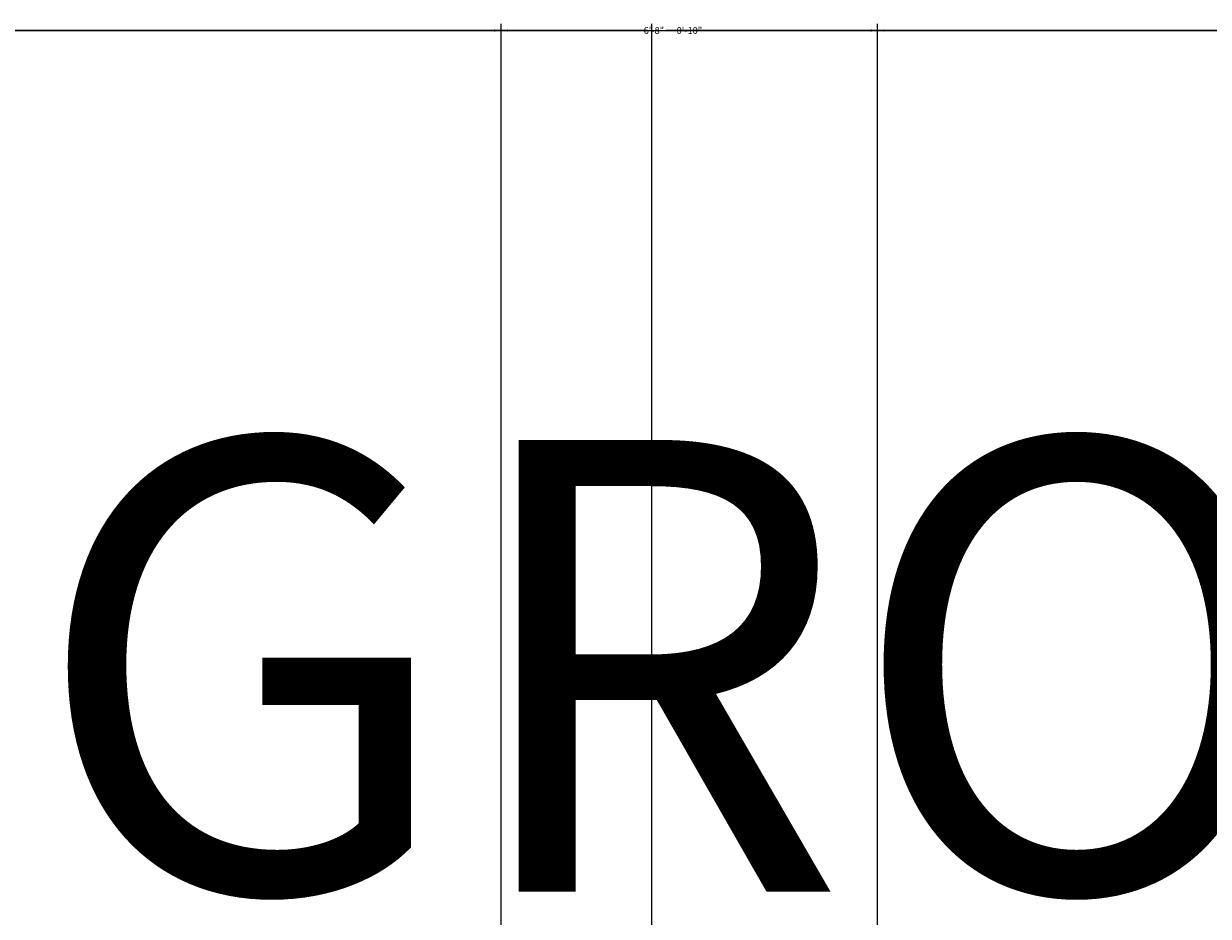
# Model space of a CAD drawing. Units: inches. Extents: x 37 to 824, y -700 to 234.
# Tile 59 of 77: x 193 to 225, y 210 to 234. Entities that reach past the tile are written whole.
import ezdxf

# ---------------------------------------------------------------- set-up
doc = ezdxf.new("R2010")
doc.units = ezdxf.units.IN
doc.header["$MEASUREMENT"] = 0
doc.layers.add('A-ANNO-DIMS', color=2, linetype='Continuous', lineweight=18)
doc.layers.add('A-ANNO-TEXT', color=7, linetype='Continuous', lineweight=18)
doc.styles.get("Standard").update_dxf_attribs({"font": 'arial.ttf'})
doc.dimstyles.get("Standard").update_dxf_attribs({"dimtxt": 0.18, "dimasz": 0.18, "dimexe": 0.18, "dimexo": 0.0625, "dimgap": 0.09, "dimtad": 0, "dimtih": 1, "dimtoh": 1, "dimdec": 1, "dimzin": 0, "dimdsep": 46, "dimlunit": 4, "dimtxsty": 'Standard', "dimcen": 0.09, "dimadec": 0, "dimazin": 0, "dimtfac": 1, "dimtdec": 1, "dimtofl": 0, "dimtmove": 0, "dimatfit": 3, "dimfxl": 1, "dimtolj": 1, "dimtzin": 0, "dimarcsym": 0})

# ---------------------------------------------------------------- blocks, each defined once
blk = doc.blocks.new('*D44')
at = {"layer": 'A-ANNO-DIMS', "color": 0, "lineweight": -2, "ltscale": 0.5, "transparency": 16777216}
for p, q in [((161.077, 191.153), (161.077, 234.17)), ((210.077, 191.153), (210.077, 234.17)), ((161.257, 233.99), (185.244, 233.99)), ((209.897, 233.99), (185.91, 233.99))]:
    blk.add_line(p, q, dxfattribs=at)
at = {"layer": 'A-ANNO-DIMS', "color": 0, "ltscale": 0.5, "transparency": 16777216}
for points in [[(161.257, 234.02), (161.257, 233.96), (161.077, 233.99)], [(209.897, 234.02), (209.897, 233.96), (210.077, 233.99)]]:
    blk.add_solid(points, dxfattribs=at)
at = {"layer": 'Defpoints', "color": 0, "ltscale": 0.5, "transparency": 16777216}
for p in [(210.077, 233.99), (161.077, 191.09), (210.077, 191.09)]:
    blk.add_point(p, dxfattribs=at)
at = {"layer": 'A-ANNO-DIMS', "color": 0, "ltscale": 0.5, "transparency": 16777216, "insert": (185.577, 233.99), "char_height": 0.18, "attachment_point": 5}
blk.add_mtext('\\A1;4\'-1"', dxfattribs=at)
blk = doc.blocks.new('*D45')
at = {"layer": 'A-ANNO-DIMS', "color": 0, "lineweight": -2, "ltscale": 0.5, "transparency": 16777216}
for p, q in [((210.077, 191.153), (210.077, 234.17)), ((250.077, 191.153), (250.077, 234.17)), ((210.257, 233.99), (229.748, 233.99)), ((249.897, 233.99), (230.406, 233.99))]:
    blk.add_line(p, q, dxfattribs=at)
at = {"layer": 'A-ANNO-DIMS', "color": 0, "ltscale": 0.5, "transparency": 16777216}
for points in [[(210.257, 234.02), (210.257, 233.96), (210.077, 233.99)], [(249.897, 234.02), (249.897, 233.96), (250.077, 233.99)]]:
    blk.add_solid(points, dxfattribs=at)
at = {"layer": 'Defpoints', "color": 0, "ltscale": 0.5, "transparency": 16777216}
for p in [(250.077, 233.99), (210.077, 191.09), (250.077, 191.09)]:
    blk.add_point(p, dxfattribs=at)
at = {"layer": 'A-ANNO-DIMS', "color": 0, "ltscale": 0.5, "transparency": 16777216, "insert": (230.077, 233.99), "char_height": 0.18, "attachment_point": 5}
blk.add_mtext('\\A1;3\'-4"', dxfattribs=at)
blk = doc.blocks.new('*D63')
at = {"layer": 'A-ANNO-DIMS', "color": 0, "lineweight": -2, "ltscale": 0.5, "transparency": 16777216}
for p, q in [((161.077, 191.153), (161.077, 234.17)), ((428.077, 191.153), (428.077, 234.17)), ((161.257, 233.99), (294.176, 233.99)), ((427.897, 233.99), (294.978, 233.99))]:
    blk.add_line(p, q, dxfattribs=at)
at = {"layer": 'A-ANNO-DIMS', "color": 0, "ltscale": 0.5, "transparency": 16777216}
for points in [[(161.257, 234.02), (161.257, 233.96), (161.077, 233.99)], [(427.897, 234.02), (427.897, 233.96), (428.077, 233.99)]]:
    blk.add_solid(points, dxfattribs=at)
at = {"layer": 'Defpoints', "color": 0, "ltscale": 0.5, "transparency": 16777216}
for p in [(428.077, 233.99), (161.077, 191.09), (428.077, 191.09)]:
    blk.add_point(p, dxfattribs=at)
at = {"layer": 'A-ANNO-DIMS', "color": 0, "ltscale": 0.5, "transparency": 16777216, "insert": (294.577, 233.99), "char_height": 0.18, "attachment_point": 5}
blk.add_mtext('\\A1;22\'-3"', dxfattribs=at)
blk = doc.blocks.new('*D72')
at = {"layer": 'A-ANNO-DIMS', "color": 0, "lineweight": -2, "ltscale": 0.5, "transparency": 16777216}
for p, q in [((170.077, 84.153), (170.077, 234.17)), ((250.19, 84.153), (250.19, 234.17)), ((170.257, 233.99), (209.804, 233.99)), ((250.01, 233.99), (210.463, 233.99))]:
    blk.add_line(p, q, dxfattribs=at)
at = {"layer": 'A-ANNO-DIMS', "color": 0, "ltscale": 0.5, "transparency": 16777216}
for points in [[(170.257, 234.02), (170.257, 233.96), (170.077, 233.99)], [(250.01, 234.02), (250.01, 233.96), (250.19, 233.99)]]:
    blk.add_solid(points, dxfattribs=at)
at = {"layer": 'Defpoints', "color": 0, "ltscale": 0.5, "transparency": 16777216}
for p in [(250.19, 233.99), (170.077, 84.09), (250.19, 84.09)]:
    blk.add_point(p, dxfattribs=at)
at = {"layer": 'A-ANNO-DIMS', "color": 0, "ltscale": 0.5, "transparency": 16777216, "insert": (210.133, 233.99), "char_height": 0.18, "attachment_point": 5}
blk.add_mtext('\\A1;6\'-8"', dxfattribs=at)
blk = doc.blocks.new('*D84')
at = {"layer": 'A-ANNO-DIMS', "color": 0, "lineweight": -2, "ltscale": 0.5, "transparency": 16777216}
for p, q in [((170.077, -265.847), (170.077, 234.17)), ((210.077, -265.847), (210.077, 234.17)), ((170.257, 233.99), (189.748, 233.99)), ((209.897, 233.99), (190.406, 233.99))]:
    blk.add_line(p, q, dxfattribs=at)
at = {"layer": 'A-ANNO-DIMS', "color": 0, "ltscale": 0.5, "transparency": 16777216}
for points in [[(170.257, 234.02), (170.257, 233.96), (170.077, 233.99)], [(209.897, 234.02), (209.897, 233.96), (210.077, 233.99)]]:
    blk.add_solid(points, dxfattribs=at)
at = {"layer": 'Defpoints', "color": 0, "ltscale": 0.5, "transparency": 16777216}
for p in [(210.077, 233.99), (170.077, -265.91), (210.077, -265.91)]:
    blk.add_point(p, dxfattribs=at)
at = {"layer": 'A-ANNO-DIMS', "color": 0, "ltscale": 0.5, "transparency": 16777216, "insert": (190.077, 233.99), "char_height": 0.18, "attachment_point": 5}
blk.add_mtext('\\A1;3\'-4"', dxfattribs=at)
blk = doc.blocks.new('*D85')
at = {"layer": 'A-ANNO-DIMS', "color": 0, "lineweight": -2, "ltscale": 0.5, "transparency": 16777216}
for p, q in [((170.077, -356.847), (170.077, 234.17)), ((206.077, -356.847), (206.077, 234.17)), ((170.257, 233.99), (187.748, 233.99)), ((205.897, 233.99), (188.406, 233.99))]:
    blk.add_line(p, q, dxfattribs=at)
at = {"layer": 'A-ANNO-DIMS', "color": 0, "ltscale": 0.5, "transparency": 16777216}
for points in [[(170.257, 234.02), (170.257, 233.96), (170.077, 233.99)], [(205.897, 234.02), (205.897, 233.96), (206.077, 233.99)]]:
    blk.add_solid(points, dxfattribs=at)
at = {"layer": 'Defpoints', "color": 0, "ltscale": 0.5, "transparency": 16777216}
for p in [(206.077, 233.99), (170.077, -356.91), (206.077, -356.91)]:
    blk.add_point(p, dxfattribs=at)
at = {"layer": 'A-ANNO-DIMS', "color": 0, "ltscale": 0.5, "transparency": 16777216, "insert": (188.077, 233.99), "char_height": 0.18, "attachment_point": 5}
blk.add_mtext('\\A1;3\'-0"', dxfattribs=at)
blk = doc.blocks.new('*D86')
at = {"layer": 'A-ANNO-DIMS', "color": 0, "lineweight": -2, "ltscale": 0.5, "transparency": 16777216}
for p, q in [((206.077, -356.847), (206.077, 234.17)), ((216.077, -356.847), (216.077, 234.17)), ((206.257, 233.99), (210.678, 233.99)), ((215.897, 233.99), (211.476, 233.99))]:
    blk.add_line(p, q, dxfattribs=at)
at = {"layer": 'A-ANNO-DIMS', "color": 0, "ltscale": 0.5, "transparency": 16777216}
for points in [[(206.257, 234.02), (206.257, 233.96), (206.077, 233.99)], [(215.897, 234.02), (215.897, 233.96), (216.077, 233.99)]]:
    blk.add_solid(points, dxfattribs=at)
at = {"layer": 'Defpoints', "color": 0, "ltscale": 0.5, "transparency": 16777216}
for p in [(216.077, 233.99), (206.077, -356.91), (216.077, -356.91)]:
    blk.add_point(p, dxfattribs=at)
at = {"layer": 'A-ANNO-DIMS', "color": 0, "ltscale": 0.5, "transparency": 16777216, "insert": (211.077, 233.99), "char_height": 0.18, "attachment_point": 5}
blk.add_mtext('\\A1;0\'-10"', dxfattribs=at)
blk = doc.blocks.new('*D87')
at = {"layer": 'A-ANNO-DIMS', "color": 0, "lineweight": -2, "ltscale": 0.5, "transparency": 16777216}
for p, q in [((216.077, -356.847), (216.077, 234.17)), ((296.077, -356.847), (296.077, 234.17)), ((216.257, 233.99), (255.747, 233.99)), ((295.897, 233.99), (256.407, 233.99))]:
    blk.add_line(p, q, dxfattribs=at)
at = {"layer": 'A-ANNO-DIMS', "color": 0, "ltscale": 0.5, "transparency": 16777216}
for points in [[(216.257, 234.02), (216.257, 233.96), (216.077, 233.99)], [(295.897, 234.02), (295.897, 233.96), (296.077, 233.99)]]:
    blk.add_solid(points, dxfattribs=at)
at = {"layer": 'Defpoints', "color": 0, "ltscale": 0.5, "transparency": 16777216}
for p in [(296.077, 233.99), (216.077, -356.91), (296.077, -356.91)]:
    blk.add_point(p, dxfattribs=at)
at = {"layer": 'A-ANNO-DIMS', "color": 0, "ltscale": 0.5, "transparency": 16777216, "insert": (256.077, 233.99), "char_height": 0.18, "attachment_point": 5}
blk.add_mtext('\\A1;6\'-8"', dxfattribs=at)

msp = doc.modelspace()

# ---------------------------------------------------------------- texts
at = {"layer": 'A-ANNO-TEXT'}
msp.add_text('GROUND  FLOOR  PLAN', height=12, dxfattribs=at).set_placement((193.612, 211.117))

# ---------------------------------------------------------------- dimensions: what is measured, and where the dimension line sits
at = {"layer": 'A-ANNO-DIMS', "ltscale": 0.5}
for base, p1, p2, picture, middle in [((210.077, 233.99), (161.077, 191.09), (210.077, 191.09), '*D44', (185.577, 233.99)), ((428.077, 233.99), (161.077, 191.09), (428.077, 191.09), '*D63', (294.577, 233.99)), ((250.19, 233.99), (170.077, 84.09), (250.19, 84.09), '*D72', (210.133, 233.99)), ((210.077, 233.99), (170.077, -265.91), (210.077, -265.91), '*D84', (190.077, 233.99)), ((206.077, 233.99), (170.077, -356.91), (206.077, -356.91), '*D85', (188.077, 233.99)), ((216.077, 233.99), (206.077, -356.91), (216.077, -356.91), '*D86', (211.077, 233.99)), ((250.077, 233.99), (210.077, 191.09), (250.077, 191.09), '*D45', (230.077, 233.99)), ((296.077, 233.99), (216.077, -356.91), (296.077, -356.91), '*D87', (256.077, 233.99))]:
    dim = msp.add_linear_dim(base=base, p1=p1, p2=p2, dimstyle='Standard', override={"dimdec": 1, "dimlfac": 1, "dimrnd": 0, "dimzin": 1, "dimdsep": 46, "dimlunit": 4, "dimfrac": 2}, dxfattribs=at)
    dim.commit()
    dim.dimension.update_dxf_attribs({"geometry": picture, "text_midpoint": middle})

doc.saveas('drawing.dxf')
